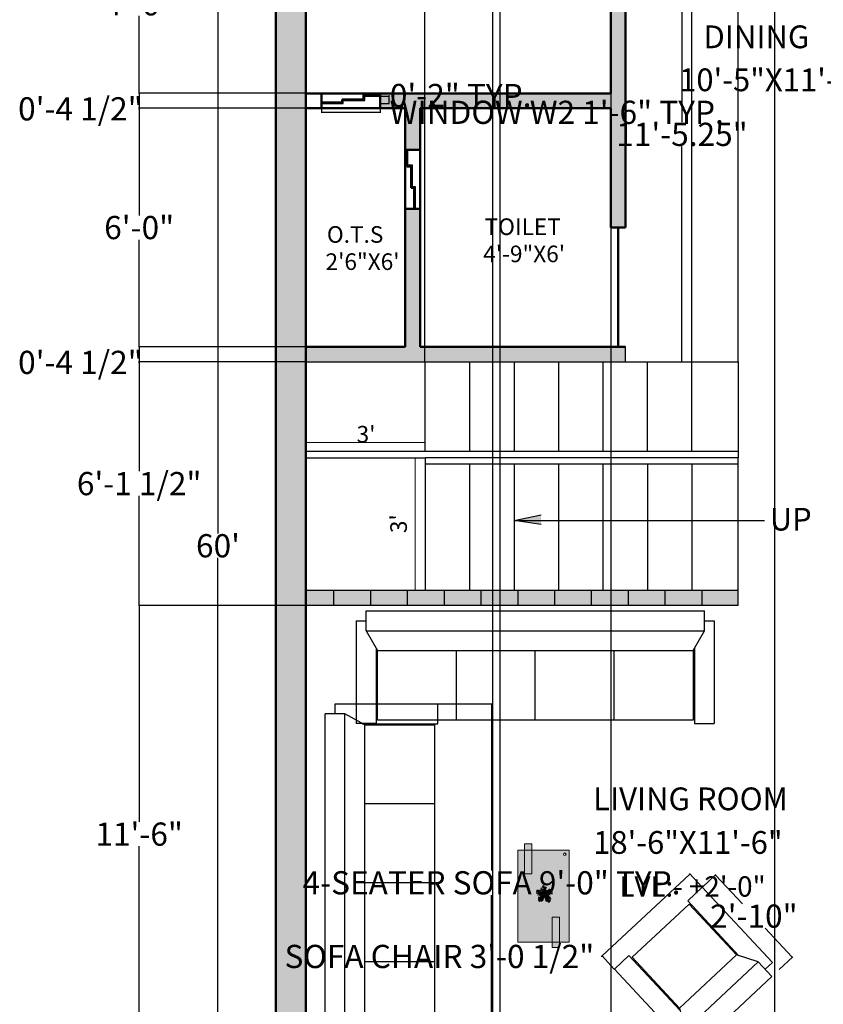
# Model space of a CAD drawing. Units: inches. Extents: x 48 to 822, y -191 to 651.
# Tile 5 of 13: x 48 to 291, y 101 to 398. Entities that reach past the tile are written whole.
import ezdxf

# ---------------------------------------------------------------- set-up
doc = ezdxf.new("R2010")
doc.units = ezdxf.units.IN
doc.header["$MEASUREMENT"] = 0
doc.layers.get('0').update_dxf_attribs({"color": 254})
for name, color, linetype, lineweight in [('A-ANNO-DIMS', 2, 'Continuous', 18), ('A-ANNO-TEXT', 3, 'Continuous', 25), ('A-AREA-IDEN', 7, 'Continuous', 25), ('A-FLOR-STRS', 3, 'Continuous', 25), ('A-FURN', 8, 'Continuous', 18), ('A-GLAZ', 4, 'Continuous', 25), ('A-WALL', 7, 'Continuous', 50), ('A-WALL-PATT', 8, 'Continuous', 13), ('L-PLNT', 103, 'Continuous', 18)]:
    doc.layers.add(name, color=color, linetype=linetype, lineweight=lineweight)
doc.layers.add('furniture', color=250, linetype='Continuous')
doc.styles.get("Standard").update_dxf_attribs({"font": 'arial.ttf'})
doc.dimstyles.get("Standard").update_dxf_attribs({"dimtxt": 7, "dimasz": 0.18, "dimexe": 0.18, "dimexo": 0.0625, "dimgap": 0.09, "dimtad": 0, "dimtih": 1, "dimtoh": 1, "dimzin": 0, "dimdsep": 46, "dimlunit": 3, "dimtxsty": 'Standard', "dimcen": 0.09, "dimadec": 0, "dimazin": 0, "dimtfac": 1, "dimtofl": 0, "dimtmove": 0, "dimatfit": 3, "dimfxl": 1, "dimtolj": 1, "dimtzin": 0, "dimarcsym": 0})

# ---------------------------------------------------------------- blocks, each defined once
blk = doc.blocks.new('FABRIC SOFA 1S')
at = {"layer": 'furniture'}
for p, q in [((3, 18.12), (34, 18.12)), ((3, 15.12), (3, 18.12)), ((34, 12.12), (34, 18.12)), ((0, -15.12), (0, 15.12)), ((6, 15.12), (0, 15.12)), ((6, -15.12), (6, 15.12)), ((12, 11.75), (6, 15.12)), ((11.33, 12.12), (34, 12.12)), ((6, -15.12), (12, -11.75)), ((11.33, -12.12), (34, -12.12)), ((34, -12.12), (34, -18.12)), ((6, -15.12), (0, -15.12)), ((3, -18.12), (3, -15.12)), ((3, -18.12), (34, -18.12))]:
    blk.add_line(p, q, dxfattribs=at)
blk.add_lwpolyline([(12, -11.75), (12, 11.75), (33, 11.75), (33, -11.75)], close=True, dxfattribs=at)
blk = doc.blocks.new('FABRIC SOFA 4S')
at = {"layer": 'furniture'}
for p, q in [((3, 54), (34, 54)), ((3, 51), (3, 54)), ((34, 48), (34, 54)), ((0, -51), (0, 51)), ((6, 51), (0, 51)), ((6, -51), (6, 51)), ((12, 47.63), (6, 51)), ((11.14, 48), (34, 48)), ((33, 23.81), (12, 23.81)), ((33, 0), (12, 0)), ((33, -23.81), (12, -23.81)), ((6, -51), (12, -47.63)), ((11.54, -48), (34, -48)), ((34, -48), (34, -54)), ((6, -51), (0, -51)), ((3, -54), (3, -51)), ((3, -54), (34, -54))]:
    blk.add_line(p, q, dxfattribs=at)
blk.add_lwpolyline([(12, -47.63), (12, 47.63), (33, 47.63), (33, -47.63)], close=True, dxfattribs=at)
blk = doc.blocks.new('*U15')
for p, q in [((-47.498, 19.737), (-55.83, 18.344)), ((-40.615, 13.7), (-55.105, 10.913)), ((-31.5, 4.5), (-52.5, 25.5)), ((-33.37, 6.269), (-52.207, 5.34)), ((-48.585, 21.131), (-49.309, 29.026)), ((-28.299, 3.483), (-47.86, -5.805)), ((-43.513, 28.561), (-42.427, 15.558)), ((-38.442, 26.239), (-34.819, 7.663)), ((-21.416, 3.018), (-38.079, -8.128)), ((-35.544, 28.097), (-24.314, 3.947)), ((0, 0), (-31.5, 4.5)), ((-14.533, 2.09), (-30.834, 25.31)), ((-15.982, 2.09), (-30.11, -9.521)), ((-3.665, 19.273), (-27.574, 35.527)), ((-5.114, 28.097), (-24.676, 40.636)), ((-24.314, 23.917), (-2.941, 13.7)), ((0, 0), (-22.5, -19.5)), ((-7.288, 39.707), (-21.778, 46.673)), ((-6.563, 1.161), (-21.416, -8.128)), ((-20.691, 13.7), (-1.129, 4.876)), ((-8.737, 47.138), (-17.069, 52.711)), ((-10.186, 53.64), (-13.084, 55.962)), ((0, 0), (-10.5, 57)), ((-9.099, 51.782), (-6.563, 55.962)), ((-7.65, 43.423), (-2.578, 49.46)), ((-5.839, 35.992), (4.667, 48.067)), ((-5.114, 27.632), (10.463, 46.673)), ((-2.941, 16.486), (8.652, 37.85)), ((-1.129, 6.734), (9.014, 26.704)), ((0, 0), (27, 9)), ((0, 0), (18, -22.5)), ((3.942, 1.625), (11.187, 24.381)), ((6.478, 1.625), (26.04, -8.592)), ((10.101, 3.483), (17.708, 26.239)), ((11.187, 3.483), (30.749, -5.805)), ((16.259, 5.805), (23.142, 31.348)), ((18.07, 5.805), (35.096, -3.483)), ((22.055, 7.198), (27.489, 32.277)), ((24.229, 7.663), (46.688, 1.625)), ((27, 9), (48, 36)), ((27.127, 9.056), (31.112, 35.992)), ((29.662, 12.307), (48.137, 6.269)), ((31.836, 30.883), (32.561, 16.486)), ((33.285, 16.486), (48.862, 10.913)), ((35.096, 32.741), (37.27, 22.524)), ((36.183, 19.737), (48.137, 17.88)), ((38.719, 34.134), (41.979, 28.561)), ((40.53, 25.775), (48.862, 24.846)), ((43.791, 29.954), (51.036, 30.883)), ((44.153, 36.456), (45.239, 32.741)), ((-17.431, -15.094), (-42.789, -18.809)), ((-28.299, -29.026), (-42.789, -31.348)), ((-24.314, -21.596), (-42.427, -22.06)), ((-30.834, -34.135), (-42.427, -35.528)), ((-34.457, -39.708), (-40.978, -42.494)), ((-26.849, -26.24), (-40.253, -25.775)), ((-22.5, -19.5), (-37.5, -45)), ((-32.646, -36.921), (-31.921, -44.352)), ((-15.257, -12.772), (-30.11, -12.772)), ((-29.023, -30.884), (-27.936, -43.887)), ((-25.038, -23.918), (-22.865, -45.281)), ((-20.691, -18.345), (-17.793, -44.352)), ((-6.563, -5.805), (-19.967, -9.985)), ((-17.069, -15.094), (-12.721, -40.172)), ((-13.446, -11.378), (-8.737, -32.741)), ((-9.461, -8.592), (-6.201, -23.453)), ((-4.752, -3.483), (-3.665, -14.629)), ((2.493, -3.019), (-1.491, -20.202)), ((1.769, -2.555), (24.229, -9.521)), ((5.029, -6.27), (2.131, -25.775)), ((9.014, -11.378), (3.58, -35.992)), ((14.085, -16.951), (6.478, -40.172)), ((7.565, -9.056), (32.198, -14.629)), ((18.07, -22.524), (8.289, -45.745)), ((12.274, -15.094), (36.907, -18.809)), ((20.244, -30.419), (15.897, -44.816)), ((16.259, -19.738), (36.183, -22.989)), ((18, -22.5), (27, -52.5)), ((18.433, -22.524), (40.53, -29.026)), ((19.157, -25.311), (38.719, -33.206)), ((22.78, -37.85), (19.519, -48.532)), ((21.331, -32.741), (39.081, -40.636)), ((22.78, -38.314), (34.372, -44.816)), ((24.591, -45.745), (23.142, -50.854)), ((24.591, -43.423), (30.749, -47.603)), ((26.764, -49.925), (28.213, -50.854))]:
    blk.add_line(p, q)
blk = doc.blocks.new('*D17')
at = {"layer": 'A-ANNO-DIMS', "color": 0, "lineweight": -2, "transparency": 16777216}
for p, q in [((109.06, 599.69), (107.79, 599.69)), ((107.97, 599.51), (107.97, 243.35)), ((107.97, -120.13), (107.97, 236.02)), ((109.06, -120.31), (107.79, -120.31))]:
    blk.add_line(p, q, dxfattribs=at)
at = {"layer": 'A-ANNO-DIMS', "color": 0, "transparency": 16777216}
for points in [[(107.94, 599.51), (108, 599.51), (107.97, 599.69)], [(107.94, -120.13), (108, -120.13), (107.97, -120.31)]]:
    blk.add_solid(points, dxfattribs=at)
at = {"layer": 'Defpoints', "color": 0, "transparency": 16777216}
for p in [(109.12, 599.69), (107.97, -120.31), (109.12, -120.31)]:
    blk.add_point(p, dxfattribs=at)
at = {"layer": 'A-ANNO-DIMS', "color": 0, "transparency": 16777216, "insert": (107.97, 239.69), "char_height": 7, "attachment_point": 5}
blk.add_mtext("\\A1;60'", dxfattribs=at)
blk = doc.blocks.new('*D20')
at = {"layer": 'A-ANNO-DIMS', "color": 0, "lineweight": -2, "transparency": 16777216}
for p, q in [((247.94, 432.26), (247.94, 367.48)), ((248, 432.44), (248.12, 432.44)), ((247.94, 295.37), (247.94, 360.15)), ((248, 295.19), (248.12, 295.19))]:
    blk.add_line(p, q, dxfattribs=at)
at = {"layer": 'A-ANNO-DIMS', "color": 0, "transparency": 16777216}
for points in [[(247.91, 432.26), (247.97, 432.26), (247.94, 432.44)], [(247.91, 295.37), (247.97, 295.37), (247.94, 295.19)]]:
    blk.add_solid(points, dxfattribs=at)
at = {"layer": 'Defpoints', "color": 0, "transparency": 16777216}
for p in [(247.94, 432.44), (247.94, 432.44), (247.94, 295.19)]:
    blk.add_point(p, dxfattribs=at)
at = {"layer": 'A-ANNO-DIMS', "color": 0, "transparency": 16777216, "insert": (247.94, 363.81), "char_height": 7, "attachment_point": 5}
blk.add_mtext('\\A1;11\'-5.25"', dxfattribs=at)
blk = doc.blocks.new('WIN-450')
for p, q in [((152.3, 373.99), (152.3, 375.35)), ((152.3, 375.35), (156.91, 375.35)), ((139.16, 373.13), (145.74, 373.13)), ((145.74, 373.13), (145.74, 373.99)), ((145.74, 373.99), (152.3, 373.99))]:
    blk.add_line(p, q)
blk = doc.blocks.new('COFFEE-TABLE')
for p, q in [((0, 27.69), (0, 0)), ((15.53, 27.69), (0, 27.69)), ((15.53, 0), (15.53, 27.69)), ((0, 0), (15.53, 0))]:
    blk.add_line(p, q)
blk = doc.blocks.new('*D30')
at = {"layer": 'A-ANNO-DIMS', "color": 0, "lineweight": -2, "transparency": 16777216}
for p, q in [((174.35, 192), (190.67, 192)), ((190.49, 191.82), (190.49, 141.72)), ((190.49, 84.18), (190.49, 134.29)), ((174.35, 84), (190.67, 84))]:
    blk.add_line(p, q, dxfattribs=at)
at = {"layer": 'A-ANNO-DIMS', "color": 0, "transparency": 16777216}
for points in [[(190.46, 191.82), (190.52, 191.82), (190.49, 192)], [(190.46, 84.18), (190.52, 84.18), (190.49, 84)]]:
    blk.add_solid(points, dxfattribs=at)
at = {"layer": 'Defpoints', "color": 0, "transparency": 16777216}
for p in [(174.29, 192), (190.49, 192), (174.29, 84)]:
    blk.add_point(p, dxfattribs=at)
at = {"layer": 'A-ANNO-DIMS', "color": 0, "transparency": 16777216, "insert": (190.49, 138), "char_height": 7, "attachment_point": 5}
blk.add_mtext('\\A1;4-SEATER SOFA 9\'-0" TYP.', dxfattribs=at)
blk = doc.blocks.new('*D36')
at = {"layer": 'A-ANNO-DIMS', "color": 0, "lineweight": -2, "transparency": 16777216}
for p, q in [((139.16, 373.06), (139.16, 370.28)), ((156.91, 373.06), (156.91, 370.28)), ((139.34, 370.46), (156.73, 370.46)), ((156.91, 370.46), (157.09, 370.46))]:
    blk.add_line(p, q, dxfattribs=at)
at = {"layer": 'A-ANNO-DIMS', "color": 0, "transparency": 16777216}
for points in [[(139.34, 370.49), (139.34, 370.43), (139.16, 370.46)], [(156.73, 370.49), (156.73, 370.43), (156.91, 370.46)]]:
    blk.add_solid(points, dxfattribs=at)
at = {"layer": 'Defpoints', "color": 0, "transparency": 16777216}
for p in [(139.16, 373.13), (156.91, 373.13), (156.91, 370.46)]:
    blk.add_point(p, dxfattribs=at)
at = {"layer": 'A-ANNO-DIMS', "color": 0, "transparency": 16777216, "insert": (210.16, 370.46), "char_height": 7, "attachment_point": 5}
blk.add_mtext('\\A1;WINDOW W2 1\'-6" TYP.', dxfattribs=at)
blk = doc.blocks.new('*D37')
at = {"layer": 'A-ANNO-DIMS', "color": 0, "lineweight": -2, "transparency": 16777216}
for p, q in [((156.97, 375.35), (159.75, 375.35)), ((159.57, 375.35), (159.57, 375.53)), ((159.57, 375.53), (159.75, 375.53)), ((159.57, 373.31), (159.57, 375.17)), ((156.97, 373.13), (159.75, 373.13))]:
    blk.add_line(p, q, dxfattribs=at)
at = {"layer": 'A-ANNO-DIMS', "color": 0, "transparency": 16777216}
for points in [[(159.54, 375.17), (159.6, 375.17), (159.57, 375.35)], [(159.54, 373.31), (159.6, 373.31), (159.57, 373.13)]]:
    blk.add_solid(points, dxfattribs=at)
at = {"layer": 'Defpoints', "color": 0, "transparency": 16777216}
for p in [(156.91, 375.35), (159.57, 375.35), (156.91, 373.13)]:
    blk.add_point(p, dxfattribs=at)
at = {"layer": 'A-ANNO-DIMS', "color": 0, "transparency": 16777216, "insert": (181.18, 375.53), "char_height": 7, "attachment_point": 5}
blk.add_mtext('\\A1;0\'-2" TYP.', dxfattribs=at)
blk = doc.blocks.new('*D44')
at = {"layer": 'A-ANNO-DIMS', "color": 0, "lineweight": -2, "transparency": 16777216}
for p, q in [((250.22, 140.52), (223.98, 116.03)), ((254.02, 136.71), (250.22, 140.77)), ((223.85, 115.9), (223.72, 115.78)), ((227.52, 111.97), (223.73, 116.03)), ((223.72, 115.78), (223.54, 115.78))]:
    blk.add_line(p, q, dxfattribs=at)
at = {"layer": 'A-ANNO-DIMS', "color": 0, "transparency": 16777216}
for points in [[(250.2, 140.54), (250.24, 140.49), (250.35, 140.64)], [(223.96, 116.05), (224, 116), (223.85, 115.9)]]:
    blk.add_solid(points, dxfattribs=at)
at = {"layer": 'Defpoints', "color": 0, "transparency": 16777216}
for p in [(254.06, 136.66), (223.85, 115.9), (227.56, 111.93)]:
    blk.add_point(p, dxfattribs=at)
at = {"layer": 'A-ANNO-DIMS', "color": 0, "transparency": 16777216, "insert": (174.76, 115.78), "char_height": 7, "attachment_point": 5}
blk.add_mtext('\\A1;SOFA CHAIR 3\'-0 1/2"', dxfattribs=at)
blk = doc.blocks.new('*D45')
at = {"layer": 'A-ANNO-DIMS', "color": 0, "lineweight": -2, "transparency": 16777216}
for p, q in [((254.1, 136.71), (258.16, 140.5)), ((258.16, 140.24), (266.21, 131.61)), ((281.11, 115.65), (273.05, 124.28)), ((277.3, 111.85), (281.36, 115.64))]:
    blk.add_line(p, q, dxfattribs=at)
at = {"layer": 'A-ANNO-DIMS', "color": 0, "transparency": 16777216}
for points in [[(258.18, 140.26), (258.13, 140.22), (258.03, 140.37)], [(281.13, 115.67), (281.09, 115.63), (281.23, 115.52)]]:
    blk.add_solid(points, dxfattribs=at)
at = {"layer": 'Defpoints', "color": 0, "transparency": 16777216}
for p in [(258.03, 140.37), (254.06, 136.66), (277.26, 111.81)]:
    blk.add_point(p, dxfattribs=at)
at = {"layer": 'A-ANNO-DIMS', "color": 0, "transparency": 16777216, "insert": (269.63, 127.95), "char_height": 7, "attachment_point": 5}
blk.add_mtext('\\A1;2\'-10"', dxfattribs=at)
blk = doc.blocks.new('*D73')
at = {"layer": 'A-ANNO-DIMS', "color": 0, "lineweight": -2, "transparency": 16777216}
for p, q in [((134.39, 430.19), (84.02, 430.19)), ((84.2, 430.01), (84.2, 406.85)), ((84.2, 376.37), (84.2, 399.52)), ((134.39, 376.19), (84.02, 376.19))]:
    blk.add_line(p, q, dxfattribs=at)
at = {"layer": 'A-ANNO-DIMS', "color": 0, "transparency": 16777216}
for points in [[(84.17, 430.01), (84.23, 430.01), (84.2, 430.19)], [(84.17, 376.37), (84.23, 376.37), (84.2, 376.19)]]:
    blk.add_solid(points, dxfattribs=at)
at = {"layer": 'Defpoints', "color": 0, "transparency": 16777216}
for p in [(134.45, 430.19), (84.2, 376.19), (134.45, 376.19)]:
    blk.add_point(p, dxfattribs=at)
at = {"layer": 'A-ANNO-DIMS', "color": 0, "transparency": 16777216, "insert": (84.2, 403.19), "char_height": 7, "attachment_point": 5}
blk.add_mtext('\\A1;4\'-6"', dxfattribs=at)
blk = doc.blocks.new('*D74')
at = {"layer": 'A-ANNO-DIMS', "color": 0, "lineweight": -2, "transparency": 16777216}
for p, q in [((134.39, 376.19), (84.02, 376.19)), ((84.2, 376.01), (84.2, 371.87)), ((134.39, 371.69), (84.02, 371.69)), ((84.2, 371.51), (84.02, 371.51)), ((84.2, 371.69), (84.2, 371.51))]:
    blk.add_line(p, q, dxfattribs=at)
at = {"layer": 'A-ANNO-DIMS', "color": 0, "transparency": 16777216}
for points in [[(84.17, 376.01), (84.23, 376.01), (84.2, 376.19)], [(84.17, 371.87), (84.23, 371.87), (84.2, 371.69)]]:
    blk.add_solid(points, dxfattribs=at)
at = {"layer": 'Defpoints', "color": 0, "transparency": 16777216}
for p in [(134.45, 376.19), (84.2, 371.69), (134.45, 371.69)]:
    blk.add_point(p, dxfattribs=at)
at = {"layer": 'A-ANNO-DIMS', "color": 0, "transparency": 16777216, "insert": (66.47, 371.51), "char_height": 7, "attachment_point": 5}
blk.add_mtext('\\A1;0\'-4 1/2"', dxfattribs=at)
blk = doc.blocks.new('*D75')
at = {"layer": 'A-ANNO-DIMS', "color": 0, "lineweight": -2, "transparency": 16777216}
for p, q in [((134.39, 371.69), (84.02, 371.69)), ((84.2, 371.51), (84.2, 339.35)), ((84.2, 299.87), (84.2, 332.02)), ((134.39, 299.69), (84.02, 299.69))]:
    blk.add_line(p, q, dxfattribs=at)
at = {"layer": 'A-ANNO-DIMS', "color": 0, "transparency": 16777216}
for points in [[(84.17, 371.51), (84.23, 371.51), (84.2, 371.69)], [(84.17, 299.87), (84.23, 299.87), (84.2, 299.69)]]:
    blk.add_solid(points, dxfattribs=at)
at = {"layer": 'Defpoints', "color": 0, "transparency": 16777216}
for p in [(134.45, 371.69), (84.2, 299.69), (134.45, 299.69)]:
    blk.add_point(p, dxfattribs=at)
at = {"layer": 'A-ANNO-DIMS', "color": 0, "transparency": 16777216, "insert": (84.2, 335.69), "char_height": 7, "attachment_point": 5}
blk.add_mtext('\\A1;6\'-0"', dxfattribs=at)
blk = doc.blocks.new('*D76')
at = {"layer": 'A-ANNO-DIMS', "color": 0, "lineweight": -2, "transparency": 16777216}
for p, q in [((134.39, 299.69), (84.02, 299.69)), ((84.2, 299.51), (84.2, 295.37)), ((134.39, 295.19), (84.02, 295.19)), ((84.2, 295.01), (84.02, 295.01)), ((84.2, 295.19), (84.2, 295.01))]:
    blk.add_line(p, q, dxfattribs=at)
at = {"layer": 'A-ANNO-DIMS', "color": 0, "transparency": 16777216}
for points in [[(84.17, 299.51), (84.23, 299.51), (84.2, 299.69)], [(84.17, 295.37), (84.23, 295.37), (84.2, 295.19)]]:
    blk.add_solid(points, dxfattribs=at)
at = {"layer": 'Defpoints', "color": 0, "transparency": 16777216}
for p in [(134.45, 299.69), (84.2, 295.19), (134.45, 295.19)]:
    blk.add_point(p, dxfattribs=at)
at = {"layer": 'A-ANNO-DIMS', "color": 0, "transparency": 16777216, "insert": (66.47, 295.01), "char_height": 7, "attachment_point": 5}
blk.add_mtext('\\A1;0\'-4 1/2"', dxfattribs=at)
blk = doc.blocks.new('*D77')
at = {"layer": 'A-ANNO-DIMS', "color": 0, "lineweight": -2, "transparency": 16777216}
for p, q in [((134.39, 295.19), (84.02, 295.19)), ((84.2, 295.01), (84.2, 262.15)), ((84.2, 221.87), (84.2, 254.73)), ((134.39, 221.69), (84.02, 221.69))]:
    blk.add_line(p, q, dxfattribs=at)
at = {"layer": 'A-ANNO-DIMS', "color": 0, "transparency": 16777216}
for points in [[(84.17, 295.01), (84.23, 295.01), (84.2, 295.19)], [(84.17, 221.87), (84.23, 221.87), (84.2, 221.69)]]:
    blk.add_solid(points, dxfattribs=at)
at = {"layer": 'Defpoints', "color": 0, "transparency": 16777216}
for p in [(134.45, 295.19), (84.2, 221.69), (134.45, 221.69)]:
    blk.add_point(p, dxfattribs=at)
at = {"layer": 'A-ANNO-DIMS', "color": 0, "transparency": 16777216, "insert": (84.2, 258.44), "char_height": 7, "attachment_point": 5}
blk.add_mtext('\\A1;6\'-1 1/2"', dxfattribs=at)
blk = doc.blocks.new('*D78')
at = {"layer": 'A-ANNO-DIMS', "color": 0, "lineweight": -2, "transparency": 16777216}
for p, q in [((134.39, 221.69), (84.02, 221.69)), ((84.2, 221.51), (84.2, 156.35)), ((84.2, 83.87), (84.2, 149.02)), ((134.39, 83.69), (84.02, 83.69))]:
    blk.add_line(p, q, dxfattribs=at)
at = {"layer": 'A-ANNO-DIMS', "color": 0, "transparency": 16777216}
for points in [[(84.17, 221.51), (84.23, 221.51), (84.2, 221.69)], [(84.17, 83.87), (84.23, 83.87), (84.2, 83.69)]]:
    blk.add_solid(points, dxfattribs=at)
at = {"layer": 'Defpoints', "color": 0, "transparency": 16777216}
for p in [(134.45, 221.69), (84.2, 83.69), (134.45, 83.69)]:
    blk.add_point(p, dxfattribs=at)
at = {"layer": 'A-ANNO-DIMS', "color": 0, "transparency": 16777216, "insert": (84.2, 152.69), "char_height": 7, "attachment_point": 5}
blk.add_mtext('\\A1;11\'-6"', dxfattribs=at)
blk = doc.blocks.new('*D89')
at = {"layer": 'A-ANNO-DIMS', "color": 0, "lineweight": -2, "transparency": 16777216}
for p, q in [((134.45, 295.25), (134.45, 641.12)), ((134.63, 640.94), (143.04, 640.94)), ((170.23, 640.94), (161.82, 640.94)), ((170.41, 295.25), (170.41, 641.12))]:
    blk.add_line(p, q, dxfattribs=at)
at = {"layer": 'A-ANNO-DIMS', "color": 0, "transparency": 16777216}
for points in [[(134.63, 640.97), (134.63, 640.91), (134.45, 640.94)], [(170.23, 640.97), (170.23, 640.91), (170.41, 640.94)]]:
    blk.add_solid(points, dxfattribs=at)
at = {"layer": 'Defpoints', "color": 0, "transparency": 16777216}
for p in [(170.41, 640.94), (134.45, 295.19), (170.41, 295.19)]:
    blk.add_point(p, dxfattribs=at)
at = {"layer": 'A-ANNO-DIMS', "color": 0, "transparency": 16777216, "insert": (152.43, 640.94), "char_height": 7, "attachment_point": 5}
blk.add_mtext('\\A1;3\'-0"', dxfattribs=at)
blk = doc.blocks.new('*D90')
at = {"layer": 'A-ANNO-DIMS', "color": 0, "lineweight": -2, "transparency": 16777216}
for p, q in [((250.94, 295.25), (250.94, 641.12)), ((251.12, 640.94), (264.75, 640.94)), ((264.93, 295.25), (264.93, 641.12)), ((264.93, 640.94), (265.11, 640.94))]:
    blk.add_line(p, q, dxfattribs=at)
at = {"layer": 'A-ANNO-DIMS', "color": 0, "transparency": 16777216}
for points in [[(251.12, 640.97), (251.12, 640.91), (250.94, 640.94)], [(264.75, 640.97), (264.75, 640.91), (264.93, 640.94)]]:
    blk.add_solid(points, dxfattribs=at)
at = {"layer": 'Defpoints', "color": 0, "transparency": 16777216}
for p in [(264.93, 640.94), (250.94, 295.19), (264.93, 295.19)]:
    blk.add_point(p, dxfattribs=at)
at = {"layer": 'A-ANNO-DIMS', "color": 0, "transparency": 16777216, "insert": (274.17, 640.94), "char_height": 7, "attachment_point": 5}
blk.add_mtext('\\A1;1\'-2"', dxfattribs=at)
blk = doc.blocks.new('*D91')
at = {"layer": 'A-ANNO-DIMS', "color": 0, "lineweight": -2, "transparency": 16777216}
for p, q in [((170.41, 295.25), (170.41, 641.12)), ((170.59, 640.94), (197.43, 640.94)), ((264.75, 640.94), (237.91, 640.94)), ((264.93, 295.25), (264.93, 641.12))]:
    blk.add_line(p, q, dxfattribs=at)
at = {"layer": 'A-ANNO-DIMS', "color": 0, "transparency": 16777216}
for points in [[(170.59, 640.97), (170.59, 640.91), (170.41, 640.94)], [(264.75, 640.97), (264.75, 640.91), (264.93, 640.94)]]:
    blk.add_solid(points, dxfattribs=at)
at = {"layer": 'Defpoints', "color": 0, "transparency": 16777216}
for p in [(264.93, 640.94), (170.41, 295.19), (264.93, 295.19)]:
    blk.add_point(p, dxfattribs=at)
at = {"layer": 'A-ANNO-DIMS', "color": 0, "transparency": 16777216, "insert": (217.67, 640.94), "char_height": 7, "attachment_point": 5}
blk.add_mtext('\\A1;7\'-10 1/2"', dxfattribs=at)
blk = doc.blocks.new('*D92')
at = {"layer": 'A-ANNO-DIMS', "color": 0, "lineweight": -2, "transparency": 16777216}
for p, q in [((275.91, 79.24), (275.91, 641.12)), ((276.09, 640.94), (293.48, 640.94)), ((293.66, 79.24), (293.66, 641.12)), ((293.66, 640.94), (293.84, 640.94))]:
    blk.add_line(p, q, dxfattribs=at)
at = {"layer": 'A-ANNO-DIMS', "color": 0, "transparency": 16777216}
for points in [[(276.09, 640.97), (276.09, 640.91), (275.91, 640.94)], [(293.48, 640.97), (293.48, 640.91), (293.66, 640.94)]]:
    blk.add_solid(points, dxfattribs=at)
at = {"layer": 'Defpoints', "color": 0, "transparency": 16777216}
for p in [(293.66, 640.94), (275.91, 79.18), (293.66, 79.18)]:
    blk.add_point(p, dxfattribs=at)
at = {"layer": 'A-ANNO-DIMS', "color": 0, "transparency": 16777216, "insert": (302.9, 640.94), "char_height": 7, "attachment_point": 5}
blk.add_mtext('\\A1;1\'-6"', dxfattribs=at)
blk = doc.blocks.new('*D94')
at = {"layer": 'A-ANNO-DIMS', "color": 0, "lineweight": -2, "transparency": 16777216}
for p, q in [((134.45, 83.75), (134.45, 641.12)), ((134.63, 640.94), (143.35, 640.94)), ((192.89, 640.94), (184.17, 640.94)), ((193.07, 83.75), (193.07, 641.12))]:
    blk.add_line(p, q, dxfattribs=at)
at = {"layer": 'A-ANNO-DIMS', "color": 0, "transparency": 16777216}
for points in [[(134.63, 640.97), (134.63, 640.91), (134.45, 640.94)], [(192.89, 640.97), (192.89, 640.91), (193.07, 640.94)]]:
    blk.add_solid(points, dxfattribs=at)
at = {"layer": 'Defpoints', "color": 0, "transparency": 16777216}
for p in [(193.07, 640.94), (134.45, 83.69), (193.07, 83.69)]:
    blk.add_point(p, dxfattribs=at)
at = {"layer": 'A-ANNO-DIMS', "color": 0, "transparency": 16777216, "insert": (163.76, 640.94), "char_height": 7, "attachment_point": 5}
blk.add_mtext('\\A1;4\'-10 1/2"', dxfattribs=at)
blk = doc.blocks.new('*D95')
at = {"layer": 'A-ANNO-DIMS', "color": 0, "lineweight": -2, "transparency": 16777216}
for p, q in [((226.45, 434.62), (226.45, -161.74)), ((190.77, 432.37), (190.77, -161.74)), ((190.95, -161.56), (226.27, -161.56)), ((226.45, -161.56), (226.63, -161.56))]:
    blk.add_line(p, q, dxfattribs=at)
at = {"layer": 'A-ANNO-DIMS', "color": 0, "transparency": 16777216}
for points in [[(190.95, -161.53), (190.95, -161.59), (190.77, -161.56)], [(226.27, -161.53), (226.27, -161.59), (226.45, -161.56)]]:
    blk.add_solid(points, dxfattribs=at)
at = {"layer": 'Defpoints', "color": 0, "transparency": 16777216}
for p in [(226.45, 434.69), (190.77, 432.44), (226.45, -161.56)]:
    blk.add_point(p, dxfattribs=at)
at = {"layer": 'A-ANNO-DIMS', "color": 0, "transparency": 16777216, "insert": (246.96, -161.56), "char_height": 7, "attachment_point": 5}
blk.add_mtext('\\A1;2\'-11 1/2"', dxfattribs=at)

msp = doc.modelspace()

# ---------------------------------------------------------------- hatches: boundary and pattern name
at = {"layer": 'A-FLOR-STRS'}
h = msp.add_hatch(color=256, dxfattribs=at)
h.dxf.hatch_style = 1
h.paths.add_polyline_path([(205.447, 249.006), (197.281, 247.361), (205.447, 246.084)])
at = {"layer": 'A-FURN'}
h = msp.add_hatch(color=256, dxfattribs=at)
h.dxf.hatch_style = 1
h.paths.add_polyline_path([(202.613, 147.821), (200.419, 147.821), (200.419, 140.695), (202.613, 140.695)])
h.paths.add_polyline_path([(202.613, 149.786), (200.419, 149.786), (200.419, 147.821), (202.613, 147.821)])
h.paths.add_polyline_path([(210.965, 127.599), (208.772, 127.599), (208.772, 120.128), (210.965, 120.128)])
h.paths.add_polyline_path([(210.965, 120.128), (208.772, 120.128), (208.772, 118.508), (210.965, 118.508)])
h = msp.add_hatch(color=256, dxfattribs=at)
h.dxf.hatch_style = 1
h.paths.add_polyline_path([(213.907, 147.821), (202.613, 147.821), (202.613, 140.695), (200.419, 140.695), (200.419, 147.821), (198.382, 147.821), (198.382, 120.128), (208.772, 120.128), (208.772, 127.599), (210.965, 127.599), (210.965, 120.128), (213.907, 120.128)])
h.paths.add_polyline_path([(205.865, 134.609), (205.839, 134.645), (205.805, 134.617)], flags=16)
h.paths.add_polyline_path([(204.25, 135.535), (204.977, 134.808), (204.917, 134.805), (204.902, 134.882), (204.334, 135.45), (204.259, 135.437)], flags=16)
h.paths.add_polyline_path([(207.626, 132.705), (207.625, 132.7), (207.628, 132.698)], flags=16)
h.paths.add_polyline_path([(206.322, 135.833), (206.311, 135.82), (206.552, 134.511), (207.028, 134.669), (207.037, 134.696), (207.067, 134.682), (207.83, 134.937), (208.094, 135.276), (208.093, 135.303), (208.111, 135.297), (207.837, 134.946), (207.836, 134.939), (206.552, 134.511), (206.653, 134.384), (206.673, 134.378), (206.669, 134.364), (207.122, 133.798), (207.242, 133.78), (207.212, 133.686), (207.399, 133.452), (207.409, 133.449), (207.407, 133.442), (206.552, 134.511), (205.742, 133.808), (205.744, 133.798), (205.728, 133.796), (206.552, 134.511), (206.307, 135.843)], flags=16)
h.paths.add_polyline_path([(212.152, 146.607, -1), (212.954, 146.607, -1)], flags=16)
at = {"layer": 'A-GLAZ'}
h = msp.add_hatch(color=256, dxfattribs=at)
h.dxf.hatch_style = 1
h.paths.add_polyline_path([(145.738, 373.987), (152.298, 373.987), (152.298, 375.346), (156.909, 375.346), (156.909, 375.689), (151.917, 375.689), (151.917, 374.347), (145.434, 374.347), (145.434, 373.472), (139.159, 373.472), (139.159, 373.126), (145.738, 373.126)])
h = msp.add_hatch(color=256, dxfattribs=at)
h.dxf.hatch_style = 1
h.paths.add_polyline_path([(166.651, 347.948), (166.651, 354.509), (165.291, 354.509), (165.291, 359.12), (164.949, 359.12), (164.949, 354.128), (166.291, 354.128), (166.291, 347.645), (167.166, 347.645), (167.166, 341.37), (167.511, 341.37), (167.511, 347.948)])
at = {"layer": 'A-WALL-PATT'}
h = msp.add_hatch(color=256, dxfattribs=at)
h.dxf.hatch_style = 1
h.paths.add_polyline_path([(134.451, 590.687), (267.451, 590.687), (267.451, 585.522), (271.951, 585.522), (271.951, 590.687), (356.451, 590.687), (356.451, 83.687), (348.824, 83.687), (348.824, 74.687), (365.451, 74.687), (365.451, 599.687), (125.451, 599.687), (125.451, -67.813), (171.204, -67.813), (171.204, -58.813), (134.451, -58.813), (134.451, 79.187), (193.069, 79.187), (193.069, 83.687), (134.451, 83.687), (134.451, 430.187), (190.775, 430.187), (190.775, 434.687), (134.451, 434.687)])
h.paths.add_polyline_path([(271.951, 550.72), (267.451, 550.72), (267.451, 430.187), (271.951, 430.187)], flags=17)
h.paths.add_polyline_path([(230.951, 432.437), (226.451, 432.437), (226.451, 376.187), (156.909, 376.187), (156.909, 371.687), (164.451, 371.687), (164.451, 359.12), (168.951, 359.12), (168.951, 371.687), (226.451, 371.687), (226.451, 335.687), (230.951, 335.687)], flags=17)
h.paths.add_polyline_path([(168.951, 341.37), (164.451, 341.37), (164.451, 299.687), (134.451, 299.687), (134.451, 295.187), (230.951, 295.187), (230.951, 299.687), (168.951, 299.687)], flags=17)
h.paths.add_polyline_path([(275.909, 83.687), (271.451, 83.687), (245.975, 83.687), (245.975, 79.187), (271.451, 79.187), (271.451, 15.696), (275.951, 15.696), (275.951, 79.177), (275.909, 79.177)], flags=17)
h.paths.add_polyline_path([(275.951, -40.13), (271.451, -40.13), (271.451, -58.813), (227.03, -58.813), (227.03, -67.813), (275.951, -67.813)], flags=17)
h = msp.add_hatch(color=256, dxfattribs=at)
h.dxf.hatch_style = 1
h.paths.add_polyline_path([(153.965, 226.187), (142.862, 226.187), (142.862, 221.687), (153.965, 221.687)])
h.paths.add_polyline_path([(176.172, 226.187), (165.069, 226.187), (165.069, 221.687), (176.172, 221.687)])
h.paths.add_polyline_path([(198.379, 226.187), (187.276, 226.187), (187.276, 221.687), (198.379, 221.687)])
h.paths.add_polyline_path([(220.587, 226.187), (209.483, 226.187), (209.483, 221.687), (220.587, 221.687)])
h.paths.add_polyline_path([(242.794, 226.187), (231.69, 226.187), (231.69, 221.687), (242.794, 221.687)])
h.paths.add_polyline_path([(264.927, 226.187), (253.897, 226.187), (253.897, 221.687), (264.927, 221.687)])
h.paths.add_polyline_path([(356.451, 278.684), (329.451, 278.684), (329.451, 226.187), (356.451, 226.187)])
h = msp.add_hatch(color=256, dxfattribs=at)
h.dxf.hatch_style = 1
h.paths.add_polyline_path([(253.897, 226.187), (242.794, 226.187), (242.794, 221.687), (253.897, 221.687)])
h.paths.add_polyline_path([(231.69, 226.187), (220.587, 226.187), (220.587, 221.687), (231.69, 221.687)])
h.paths.add_polyline_path([(209.483, 226.187), (198.379, 226.187), (198.379, 221.687), (209.483, 221.687)])
h.paths.add_polyline_path([(187.276, 226.187), (176.172, 226.187), (176.172, 221.687), (187.276, 221.687)])
h.paths.add_polyline_path([(165.069, 226.187), (153.965, 226.187), (153.965, 221.687), (165.069, 221.687)])
h.paths.add_polyline_path([(142.862, 226.187), (134.451, 226.187), (134.451, 221.687), (142.862, 221.687)])

# ---------------------------------------------------------------- linework, layer by layer
at = {"layer": 'A-ANNO-DIMS'}
for p, q in [((134.451, 270.836), (170.413, 270.836)), ((167.439, 266.171), (167.439, 226.187))]:
    msp.add_line(p, q, dxfattribs=at)
at = {"layer": 'A-FLOR-STRS'}
for p, q in [((230.951, 295.187), (230.951, 299.687)), ((134.451, 295.187), (230.951, 295.187)), ((170.413, 295.187), (170.413, 268.257)), ((183.866, 295.187), (183.866, 268.257)), ((197.281, 295.187), (197.281, 268.257)), ((210.696, 295.187), (210.696, 268.257)), ((224.112, 295.187), (224.112, 268.257)), ((230.951, 295.187), (264.927, 295.187)), ((237.527, 268.257), (237.527, 295.187)), ((250.942, 268.257), (250.942, 295.187)), ((264.927, 295.187), (264.927, 266.171)), ((134.451, 268.257), (264.927, 268.257)), ((134.451, 266.171), (170.451, 266.171)), ((170.451, 266.171), (170.451, 226.187)), ((264.927, 266.171), (170.451, 266.171)), ((170.451, 264.407), (264.927, 264.407)), ((183.866, 264.407), (183.866, 226.187)), ((197.281, 264.407), (197.281, 226.187)), ((210.696, 264.407), (210.696, 226.187)), ((224.112, 264.407), (224.112, 226.187)), ((237.527, 264.407), (237.527, 226.187)), ((250.942, 264.407), (250.942, 226.187)), ((264.927, 226.187), (264.927, 266.171)), ((197.281, 247.361), (205.447, 249.006)), ((197.281, 247.361), (272.855, 247.361)), ((205.447, 246.084), (197.281, 247.361)), ((264.927, 226.187), (134.451, 226.187)), ((142.862, 226.187), (142.862, 221.687)), ((153.965, 226.187), (153.965, 221.687)), ((165.069, 226.187), (165.069, 221.687)), ((176.172, 226.187), (176.172, 221.687)), ((187.276, 226.187), (187.276, 221.687)), ((198.379, 226.187), (198.379, 221.687)), ((209.483, 226.187), (209.483, 221.687)), ((220.587, 226.187), (220.587, 221.687)), ((231.69, 226.187), (231.69, 221.687)), ((242.794, 226.187), (242.794, 221.687)), ((253.897, 226.187), (253.897, 221.687)), ((264.927, 221.687), (264.927, 226.187)), ((264.927, 221.687), (134.451, 221.687))]:
    msp.add_line(p, q, dxfattribs=at)
at = {"layer": 'A-FURN'}
for p, q in [((200.419, 149.786), (202.613, 149.786)), ((200.419, 140.695), (200.419, 149.786)), ((202.613, 149.786), (202.613, 140.695)), ((202.613, 140.695), (200.419, 140.695)), ((208.772, 127.599), (210.965, 127.599)), ((208.772, 118.508), (208.772, 127.599)), ((210.965, 127.599), (210.965, 118.508)), ((210.965, 118.508), (208.772, 118.508))]:
    msp.add_line(p, q, dxfattribs=at)
msp.add_circle((212.553, 146.607), 0.401, dxfattribs=at)
at = {"layer": 'A-WALL'}
for p, q in [((125.451, -120.313), (125.451, 599.687)), ((226.451, 376.187), (226.451, 434.687)), ((230.951, 335.687), (230.951, 434.687)), ((134.451, 83.687), (134.451, 430.187)), ((134.451, 376.187), (226.451, 376.187)), ((139.159, 376.187), (139.159, 371.687)), ((156.909, 376.187), (139.159, 376.187)), ((145.434, 373.472), (145.434, 374.347)), ((145.434, 374.347), (151.917, 374.347)), ((151.917, 374.347), (151.917, 375.689)), ((151.917, 375.689), (156.909, 375.689)), ((156.909, 371.687), (156.909, 376.187)), ((134.451, 371.687), (164.451, 371.687)), ((139.159, 373.472), (145.434, 373.472)), ((139.159, 371.687), (156.909, 371.687)), ((164.451, 299.687), (164.451, 371.687)), ((168.951, 299.687), (168.951, 371.687)), ((168.951, 371.687), (226.451, 371.687)), ((226.451, 335.687), (226.451, 371.687)), ((168.951, 359.12), (164.451, 359.12)), ((164.451, 359.12), (164.451, 341.37)), ((164.949, 354.128), (164.949, 359.12)), ((168.951, 341.37), (168.951, 359.12)), ((166.291, 354.128), (164.949, 354.128)), ((166.291, 347.645), (166.291, 354.128)), ((167.166, 347.645), (166.291, 347.645)), ((167.166, 341.37), (167.166, 347.645)), ((164.451, 341.37), (168.951, 341.37)), ((226.451, 335.687), (230.951, 335.687)), ((228.701, 335.687), (228.701, 299.687)), ((134.451, 299.687), (164.451, 299.687)), ((168.951, 299.687), (230.951, 299.687))]:
    msp.add_line(p, q, dxfattribs=at)

# ---------------------------------------------------------------- block references
at = {"layer": 'A-FURN'}
for name, p, rotation in [('FABRIC SOFA 4S', (203.685, 220.048), 270), ('FABRIC SOFA 1S', (264.008, 99.441), 133.0281851586549)]:
    msp.add_blockref(name, p, dxfattribs=dict(at, rotation=rotation))
for name, p in [('FABRIC SOFA 4S', (140.286, 138.003)), ('COFFEE-TABLE', (198.382, 120.128))]:
    msp.add_blockref(name, p, dxfattribs=at)
at = {"layer": 'A-GLAZ'}
msp.add_blockref('WIN-450', (0, 0), dxfattribs=at)
at = {"layer": 'A-GLAZ', "rotation": 89.99999999999947}
msp.add_blockref('WIN-450', (540.637, 202.211), dxfattribs=at)
at = {"layer": 'L-PLNT', "xscale": 0.0473395969371584, "yscale": 0.0473395969371584, "zscale": 0.0473395969371584}
msp.add_blockref('*U15', (206.552, 134.511), dxfattribs=at)

# ---------------------------------------------------------------- texts
at = {"layer": 'A-ANNO-TEXT'}
for s, height, p in [("3'", 5.0075, (149.781, 270.836)), ('UP', 6.8277, (274.448, 244.285)), ('LVL:- +2\'-0"', 6.13413, (229.059, 133.827))]:
    msp.add_text(s, height=height, dxfattribs=at).set_placement(p)
msp.add_text("3'", height=5.0075, rotation=90, dxfattribs=at).set_placement((164.959, 243.5))
at = {"layer": 'A-AREA-IDEN'}
for s, height, p in [('DINING', 6.866, (254.419, 389.804)), ('10\'-5"X11\'-4"', 6.86603, (247.07, 376.833)), ('O.T.S', 5.0075, (140.824, 331.103)), ('TOILET', 5.0075, (188.382, 333.442)), ('4\'-9"X6\'', 5.0075, (187.978, 325.238)), ('2\'6"X6\'', 5.0075, (140.419, 322.9)), ('LIVING ROOM', 6.86603, (221.149, 159.896)), ('18\'-6"X11\'-6"', 6.86603, (221.149, 146.738))]:
    msp.add_text(s, height=height, dxfattribs=at).set_placement(p)

# ---------------------------------------------------------------- dimensions: what is measured, and where the dimension line sits
at = {"layer": 'A-ANNO-DIMS'}
for base, p1, p2, picture, middle in [((193.069, 640.937), (134.451, 83.687), (193.069, 83.687), '*D94', (163.76, 640.937)), ((264.927, 640.937), (170.413, 295.187), (264.927, 295.187), '*D91', (217.67, 640.937)), ((170.413, 640.937), (134.451, 295.187), (170.413, 295.187), '*D89', (152.432, 640.937)), ((264.927, 640.937), (250.942, 295.187), (264.927, 295.187), '*D90', (274.172, 640.937)), ((293.6592, 640.9365), (275.9088, 79.1772), (293.6592, 79.1772), '*D92', (302.9036, 640.9365)), ((226.451, -161.563), (190.775, 432.437), (226.451, 434.687), '*D95', (246.959, -161.563))]:
    dim = msp.add_linear_dim(base=base, p1=p1, p2=p2, dimstyle='Standard', override={"dimdec": 1, "dimlfac": 1, "dimrnd": 0, "dimzin": 1, "dimdsep": 46, "dimlunit": 4, "dimfrac": 2}, dxfattribs=at)
    dim.commit()
    dim.dimension.update_dxf_attribs({"geometry": picture, "text_midpoint": middle})
for base, p1, p2, angle, override, picture, middle in [((107.967, -120.313), (109.12, 599.687), (109.12, -120.313), 90, {"dimclrd": 0, "dimclre": 0, "dimclrt": 0}, '*D17', (107.967, 239.687)), ((247.939, 432.437), (247.939, 295.187), (247.939, 432.437), 90, {"dimclrd": 0, "dimclre": 0, "dimclrt": 0}, '*D20', (247.939, 363.812)), ((84.201, 376.187), (134.451, 430.187), (134.451, 376.187), 90, {"dimdec": 1, "dimlfac": 1, "dimrnd": 0, "dimzin": 1, "dimdsep": 46, "dimlunit": 4, "dimfrac": 2}, '*D73', (84.201, 403.187)), ((84.201, 371.687), (134.451, 376.187), (134.451, 371.687), 90, {"dimdec": 1, "dimlfac": 1, "dimrnd": 0, "dimzin": 1, "dimdsep": 46, "dimlunit": 4, "dimfrac": 2}, '*D74', (66.471, 371.507)), ((84.201, 299.687), (134.451, 371.687), (134.451, 299.687), 90, {"dimdec": 1, "dimlfac": 1, "dimrnd": 0, "dimzin": 1, "dimdsep": 46, "dimlunit": 4, "dimfrac": 2}, '*D75', (84.201, 335.687)), ((84.201, 295.187), (134.451, 299.687), (134.451, 295.187), 90, {"dimdec": 1, "dimlfac": 1, "dimrnd": 0, "dimzin": 1, "dimdsep": 46, "dimlunit": 4, "dimfrac": 2}, '*D76', (66.471, 295.007)), ((84.201, 221.687), (134.451, 295.187), (134.451, 221.687), 90, {"dimdec": 1, "dimlfac": 1, "dimrnd": 0, "dimzin": 1, "dimdsep": 46, "dimlunit": 4, "dimfrac": 2}, '*D77', (84.201, 258.437)), ((84.201, 83.687), (134.451, 221.687), (134.451, 83.687), 90, {"dimdec": 1, "dimlfac": 1, "dimrnd": 0, "dimzin": 1, "dimdsep": 46, "dimlunit": 4, "dimfrac": 2}, '*D78', (84.201, 152.687)), ((258.033, 140.373), (277.258, 111.808), (254.058, 136.663), 133.02819, {"dimdec": 1, "dimlfac": 1, "dimrnd": 0, "dimzin": 1, "dimdsep": 46, "dimlunit": 4, "dimfrac": 2}, '*D45', (269.633, 127.946))]:
    dim = msp.add_linear_dim(base=base, p1=p1, p2=p2, angle=angle, dimstyle='Standard', override=override, dxfattribs=at)
    dim.commit()
    dim.dimension.update_dxf_attribs({"geometry": picture, "text_midpoint": middle})
dim = msp.add_linear_dim(base=(156.9091, 370.4638), p1=(139.1587, 373.1263), p2=(156.9091, 373.1263), text='WINDOW W2 <> TYP.', dimstyle='Standard', override={"dimdec": 1, "dimlfac": 1, "dimrnd": 0, "dimzin": 1, "dimdsep": 46, "dimlunit": 4, "dimfrac": 2}, dxfattribs=at)
dim.commit()
dim.dimension.update_dxf_attribs({"geometry": '*D36', "text_midpoint": (210.1614, 370.4638)})
for base, p1, p2, angle, text, picture, middle in [((159.572, 375.346), (156.909, 373.126), (156.909, 375.346), 90, '<> TYP.', '*D37', (181.176, 375.526)), ((190.486, 192.003), (174.286, 84.003), (174.286, 192.003), 90, '4-SEATER SOFA <> TYP.', '*D30', (190.486, 138.003)), ((223.848123, 115.902529), (254.057852, 136.663097), (227.558445, 111.927618), 223.028185, 'SOFA CHAIR <>', '*D44', (174.761683, 115.779705))]:
    dim = msp.add_linear_dim(base=base, p1=p1, p2=p2, angle=angle, text=text, dimstyle='Standard', override={"dimdec": 1, "dimlfac": 1, "dimrnd": 0, "dimzin": 1, "dimdsep": 46, "dimlunit": 4, "dimfrac": 2}, dxfattribs=at)
    dim.commit()
    dim.dimension.update_dxf_attribs({"geometry": picture, "text_midpoint": middle})

doc.saveas('drawing.dxf')
